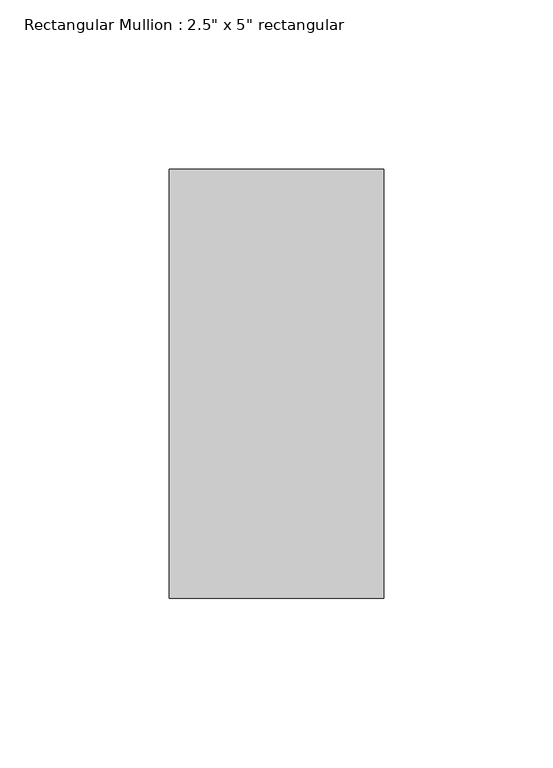
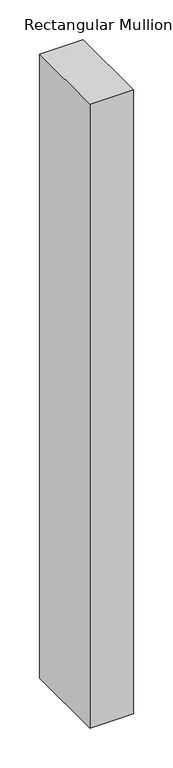
"""IFC4 building model written with IfcOpenShell, lengths in millimetres: member geometry."""

from ifc_helpers import new_model, si_unit, frame, origin, place, context, project, spatial, polyline, outline, extrude, source, transform, mapped, element, save


def member_76449a13(model_context):
    return source(origin(), model_context, "Body", "SweptSolid", [
        extrude(outline(polyline([(31.75, 63.5), (31.75, -63.5), (-31.75, -63.5), (-31.75, 63.5), (31.75, 63.5)])), frame((0.0, 0.0, -960.3935073), z_axis=(0.0, 0.0, 1.0), x_axis=(1.0, 0.0, 0.0)), (0.0, 0.0, 1.0), 960.3935073),
    ])


if __name__ == "__main__":
    model = new_model("IFC4")
    model_context = context("Model", 3, world=origin())
    ifc_project = project(units=[si_unit("LENGTHUNIT", "METRE", prefix="MILLI")], contexts=[model_context])
    site = spatial("IfcSite", under=ifc_project)
    building = spatial("IfcBuilding", under=site)
    placement = place(None, origin())
    member_shape = member_76449a13(model_context)
    element("IfcMember", 1, ObjectType="Rectangular Mullion : 2.5\" x 5\" rectangular", at=placement, inside=building, context=model_context, shape_type="MappedRepresentation", body=[
        mapped(member_shape, transform((0.0, 0.0, 0.0), x_axis=(1.0, 0.0, 0.0), y_axis=(0.0, 1.0, 0.0), z_axis=(0.0, 0.0, 1.0))),
    ])
    save(model, "model.ifc")

# Revit data of these elements
# Type "Rectangular Mullion : 2.5\" x 5\" rectangular"
#   built-in parameter 1007304 = 0.416667 (stored number, unit not read)
#   built-in parameter 1007301 = 0.104167 (stored number, unit not read)
#   built-in parameter 1007300 = 0.104167 (stored number, unit not read)
# Element 1 (IfcMember, "Rectangular Mullion : 2.5\" x 5\" rectangular")
#   Materials on its faces: "Aluminum"
# Materials
#   "Aluminum": class "Metal", colour RGB 247 247 247, transparency 0, Description = "Aluminum 6061", Cost = 0
